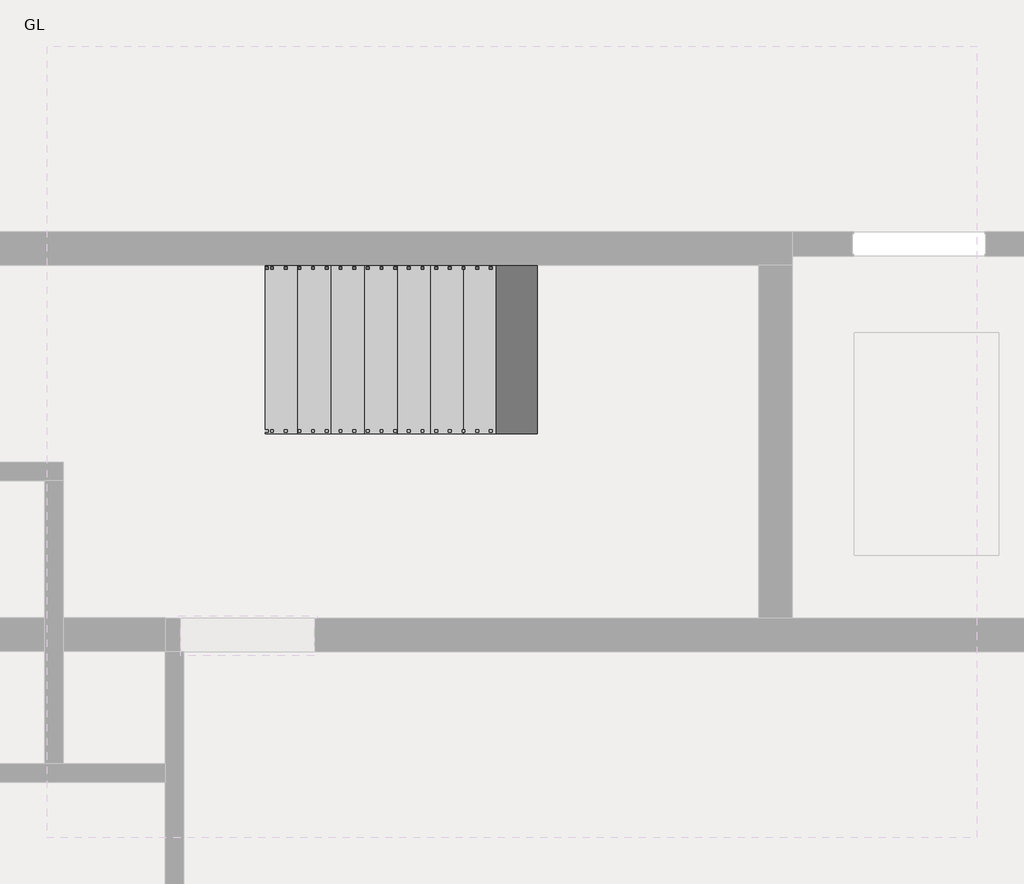
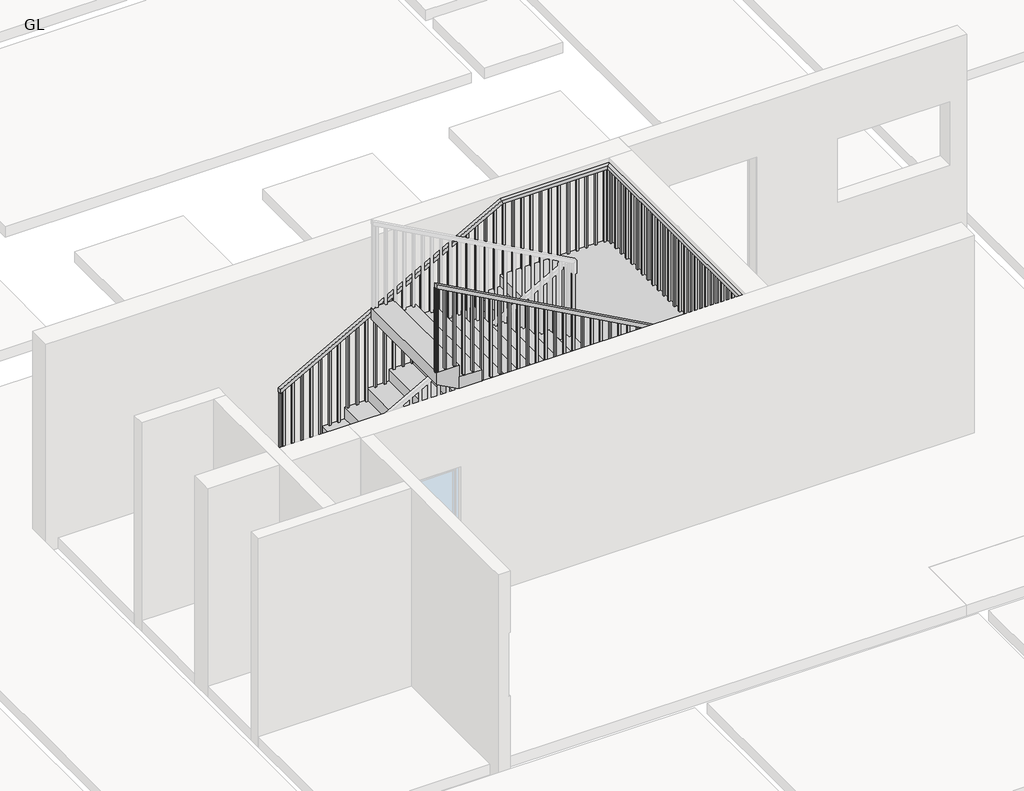
# One storey, part 10 of 14: 1 railing, 1 stair flight.
"""IFC4 building model written with IfcOpenShell, lengths in millimetres."""

from ifc_helpers import new_model, si_unit, frame, origin, place, context, project, spatial, polyline, outline, extrude, faceted_brep, element, save

model = new_model("IFC4")

# Units and contexts
model_context = context("Model", 3, world=origin())
ifc_project = project(units=[si_unit("LENGTHUNIT", "METRE", prefix="MILLI")], contexts=[model_context])

# Site, building, storey
site = spatial("IfcSite", under=ifc_project)
building = spatial("IfcBuilding", under=site)
storey = spatial("IfcBuildingStorey", under=building, Name="GL", Elevation=0.0)

# Railing
placement = place(None, origin())
element("IfcRailing", 1, ObjectType="1100mm", at=placement, inside=storey, context=model_context, shape_type="SolidModel", body=[
    faceted_brep([(-139.7980544, 73095.2178911, 1266.6666667), (-139.7980544, 73095.2178911, 1209.5692982), (-139.7980544, 73045.2178911, 1209.5692982), (-139.7980544, 73045.2178911, 1266.6666667), (2882.8019456, 73095.2178911, 2933.3333333), (2895.6734492, 73095.2178911, 2883.3333333), (2895.6734492, 73045.2178911, 2883.3333333), (2882.8019456, 73045.2178911, 2933.3333333), (4371.714024, 73095.2178911, 2933.3333333), (4371.714024, 73095.2178911, 2883.3333333), (4321.714024, 73045.2178911, 2883.3333333), (4321.714024, 73045.2178911, 2933.3333333), (4371.714024, 69866.5033979, 2933.3333333), (4371.714024, 69866.5033979, 2883.3333333), (4321.714024, 69916.5033979, 2883.3333333), (4321.714024, 69916.5033979, 2933.3333333), (3185.485279, 69866.5033979, 2933.3333333), (3172.6295437, 69866.5033979, 2883.3333333), (3172.6295437, 69916.5033979, 2883.3333333), (3185.485279, 69916.5033979, 2933.3333333), (158.6519456, 69866.5033979, 4600.0), (158.6519456, 69916.5033979, 4600.0), (158.6519456, 69916.5033979, 4542.9212405), (158.6519456, 69866.5033979, 4542.9212405)], [[[0, 1, 2, 3]], [[1, 0, 4, 5]], [[2, 1, 5, 6]], [[3, 2, 6, 7]], [[0, 3, 7, 4]], [[5, 4, 8, 9]], [[6, 5, 9, 10]], [[7, 6, 10, 11]], [[4, 7, 11, 8]], [[9, 8, 12, 13]], [[10, 9, 13, 14]], [[11, 10, 14, 15]], [[8, 11, 15, 12]], [[13, 12, 16, 17]], [[14, 13, 17, 18]], [[15, 14, 18, 19]], [[12, 15, 19, 16]], [[20, 21, 22, 23]], [[17, 16, 20, 23]], [[18, 17, 23, 22]], [[19, 18, 22, 21]], [[16, 19, 21, 20]]]),
    extrude(outline(polyline([(4535.7288621, 171.714024), (4549.4946239, 146.714024), (3333.3333333, 146.714024), (3333.3333333, 171.714024), (4535.7288621, 171.714024)])), frame((0.0, 69879.0033979, 0.0), z_axis=(0.0, 1.0, 0.0), x_axis=(0.0, 0.0, 1.0)), (0.0, 0.0, 1.0), 25.0),
    extrude(outline(polyline([(4466.9000531, 296.714024), (4480.6658149, 271.714024), (3333.3333333, 271.714024), (3333.3333333, 296.714024), (4466.9000531, 296.714024)])), frame((0.0, 69879.0033979, 0.0), z_axis=(0.0, 1.0, 0.0), x_axis=(0.0, 0.0, 1.0)), (0.0, 0.0, 1.0), 25.0),
    extrude(outline(polyline([(4398.0712441, 421.714024), (4411.8370059, 396.714024), (3333.3333333, 396.714024), (3333.3333333, 421.714024), (4398.0712441, 421.714024)])), frame((0.0, 69879.0033979, 0.0), z_axis=(0.0, 1.0, 0.0), x_axis=(0.0, 0.0, 1.0)), (0.0, 0.0, 1.0), 25.0),
    extrude(outline(polyline([(4329.2424351, 546.714024), (4343.0081969, 521.714024), (3166.6666667, 521.714024), (3166.6666667, 546.714024), (4329.2424351, 546.714024)])), frame((0.0, 69879.0033979, 0.0), z_axis=(0.0, 1.0, 0.0), x_axis=(0.0, 0.0, 1.0)), (0.0, 0.0, 1.0), 25.0),
    extrude(outline(polyline([(4260.4136261, 671.714024), (4274.1793879, 646.714024), (3166.6666667, 646.714024), (3166.6666667, 671.714024), (4260.4136261, 671.714024)])), frame((0.0, 69879.0033979, 0.0), z_axis=(0.0, 1.0, 0.0), x_axis=(0.0, 0.0, 1.0)), (0.0, 0.0, 1.0), 25.0),
    extrude(outline(polyline([(4191.5848171, 796.714024), (4205.3505789, 771.714024), (3000.0, 771.714024), (3000.0, 796.714024), (4191.5848171, 796.714024)])), frame((0.0, 69879.0033979, 0.0), z_axis=(0.0, 1.0, 0.0), x_axis=(0.0, 0.0, 1.0)), (0.0, 0.0, 1.0), 25.0),
    extrude(outline(polyline([(4122.7560081, 921.714024), (4136.5217699, 896.714024), (3000.0, 896.714024), (3000.0, 921.714024), (4122.7560081, 921.714024)])), frame((0.0, 69879.0033979, 0.0), z_axis=(0.0, 1.0, 0.0), x_axis=(0.0, 0.0, 1.0)), (0.0, 0.0, 1.0), 25.0),
    extrude(outline(polyline([(4053.9271992, 1046.714024), (4067.6929609, 1021.714024), (3000.0, 1021.714024), (3000.0, 1046.714024), (4053.9271992, 1046.714024)])), frame((0.0, 69879.0033979, 0.0), z_axis=(0.0, 1.0, 0.0), x_axis=(0.0, 0.0, 1.0)), (0.0, 0.0, 1.0), 25.0),
    extrude(outline(polyline([(3985.0983902, 1171.714024), (3998.864152, 1146.714024), (2833.3333333, 1146.714024), (2833.3333333, 1171.714024), (3985.0983902, 1171.714024)])), frame((0.0, 69879.0033979, 0.0), z_axis=(0.0, 1.0, 0.0), x_axis=(0.0, 0.0, 1.0)), (0.0, 0.0, 1.0), 25.0),
    extrude(outline(polyline([(3916.2695812, 1296.714024), (3930.035343, 1271.714024), (2833.3333333, 1271.714024), (2833.3333333, 1296.714024), (3916.2695812, 1296.714024)])), frame((0.0, 69879.0033979, 0.0), z_axis=(0.0, 1.0, 0.0), x_axis=(0.0, 0.0, 1.0)), (0.0, 0.0, 1.0), 25.0),
    extrude(outline(polyline([(3847.4407722, 1421.714024), (3861.206534, 1396.714024), (2666.6666667, 1396.714024), (2666.6666667, 1421.714024), (3847.4407722, 1421.714024)])), frame((0.0, 69879.0033979, 0.0), z_axis=(0.0, 1.0, 0.0), x_axis=(0.0, 0.0, 1.0)), (0.0, 0.0, 1.0), 25.0),
    extrude(outline(polyline([(3778.6119632, 1546.714024), (3792.377725, 1521.714024), (2666.6666667, 1521.714024), (2666.6666667, 1546.714024), (3778.6119632, 1546.714024)])), frame((0.0, 69879.0033979, 0.0), z_axis=(0.0, 1.0, 0.0), x_axis=(0.0, 0.0, 1.0)), (0.0, 0.0, 1.0), 25.0),
    extrude(outline(polyline([(3709.7831542, 1671.714024), (3723.548916, 1646.714024), (2666.6666667, 1646.714024), (2666.6666667, 1671.714024), (3709.7831542, 1671.714024)])), frame((0.0, 69879.0033979, 0.0), z_axis=(0.0, 1.0, 0.0), x_axis=(0.0, 0.0, 1.0)), (0.0, 0.0, 1.0), 25.0),
    extrude(outline(polyline([(3640.9543452, 1796.714024), (3654.720107, 1771.714024), (2500.0, 1771.714024), (2500.0, 1796.714024), (3640.9543452, 1796.714024)])), frame((0.0, 69879.0033979, 0.0), z_axis=(0.0, 1.0, 0.0), x_axis=(0.0, 0.0, 1.0)), (0.0, 0.0, 1.0), 25.0),
    extrude(outline(polyline([(3572.1255362, 1921.714024), (3585.891298, 1896.714024), (2500.0, 1896.714024), (2500.0, 1921.714024), (3572.1255362, 1921.714024)])), frame((0.0, 69879.0033979, 0.0), z_axis=(0.0, 1.0, 0.0), x_axis=(0.0, 0.0, 1.0)), (0.0, 0.0, 1.0), 25.0),
    extrude(outline(polyline([(3503.2967273, 2046.714024), (3517.0624891, 2021.714024), (2333.3333333, 2021.714024), (2333.3333333, 2046.714024), (3503.2967273, 2046.714024)])), frame((0.0, 69879.0033979, 0.0), z_axis=(0.0, 1.0, 0.0), x_axis=(0.0, 0.0, 1.0)), (0.0, 0.0, 1.0), 25.0),
    extrude(outline(polyline([(3434.4679183, 2171.714024), (3448.2336801, 2146.714024), (2333.3333333, 2146.714024), (2333.3333333, 2171.714024), (3434.4679183, 2171.714024)])), frame((0.0, 69879.0033979, 0.0), z_axis=(0.0, 1.0, 0.0), x_axis=(0.0, 0.0, 1.0)), (0.0, 0.0, 1.0), 25.0),
    extrude(outline(polyline([(3365.6391093, 2296.714024), (3379.4048711, 2271.714024), (2166.6666667, 2271.714024), (2166.6666667, 2296.714024), (3365.6391093, 2296.714024)])), frame((0.0, 69879.0033979, 0.0), z_axis=(0.0, 1.0, 0.0), x_axis=(0.0, 0.0, 1.0)), (0.0, 0.0, 1.0), 25.0),
    extrude(outline(polyline([(3296.8103003, 2421.714024), (3310.5760621, 2396.714024), (2166.6666667, 2396.714024), (2166.6666667, 2421.714024), (3296.8103003, 2421.714024)])), frame((0.0, 69879.0033979, 0.0), z_axis=(0.0, 1.0, 0.0), x_axis=(0.0, 0.0, 1.0)), (0.0, 0.0, 1.0), 25.0),
    extrude(outline(polyline([(3227.9814913, 2546.714024), (3241.7472531, 2521.714024), (2166.6666667, 2521.714024), (2166.6666667, 2546.714024), (3227.9814913, 2546.714024)])), frame((0.0, 69879.0033979, 0.0), z_axis=(0.0, 1.0, 0.0), x_axis=(0.0, 0.0, 1.0)), (0.0, 0.0, 1.0), 25.0),
    extrude(outline(polyline([(3159.1526823, 2671.714024), (3172.9184441, 2646.714024), (2000.0, 2646.714024), (2000.0, 2671.714024), (3159.1526823, 2671.714024)])), frame((0.0, 69879.0033979, 0.0), z_axis=(0.0, 1.0, 0.0), x_axis=(0.0, 0.0, 1.0)), (0.0, 0.0, 1.0), 25.0),
    extrude(outline(polyline([(3090.3238733, 2796.714024), (3104.0896351, 2771.714024), (2000.0, 2771.714024), (2000.0, 2796.714024), (3090.3238733, 2796.714024)])), frame((0.0, 69879.0033979, 0.0), z_axis=(0.0, 1.0, 0.0), x_axis=(0.0, 0.0, 1.0)), (0.0, 0.0, 1.0), 25.0),
    extrude(outline(polyline([(3021.4950644, 2921.714024), (3035.2608262, 2896.714024), (1833.3333333, 2896.714024), (1833.3333333, 2921.714024), (3021.4950644, 2921.714024)])), frame((0.0, 69879.0033979, 0.0), z_axis=(0.0, 1.0, 0.0), x_axis=(0.0, 0.0, 1.0)), (0.0, 0.0, 1.0), 25.0),
    extrude(outline(polyline([(2952.6662554, 3046.714024), (2966.4320172, 3021.714024), (1833.3333333, 3021.714024), (1833.3333333, 3046.714024), (2952.6662554, 3046.714024)])), frame((0.0, 69879.0033979, 0.0), z_axis=(0.0, 1.0, 0.0), x_axis=(0.0, 0.0, 1.0)), (0.0, 0.0, 1.0), 25.0),
    extrude(outline(polyline([(2883.8374464, 3171.714024), (2897.6032082, 3146.714024), (1833.3333333, 3146.714024), (1833.3333333, 3171.714024), (2883.8374464, 3171.714024)])), frame((0.0, 69879.0033979, 0.0), z_axis=(0.0, 1.0, 0.0), x_axis=(0.0, 0.0, 1.0)), (0.0, 0.0, 1.0), 25.0),
    extrude(outline(polyline([(3296.714024, 69879.0033979), (3271.714024, 69879.0033979), (3271.714024, 69904.0033979), (3296.714024, 69904.0033979), (3296.714024, 69879.0033979)])), frame((0.0, 0.0, 1833.3333333), z_axis=(0.0, 0.0, 1.0), x_axis=(1.0, 0.0, 0.0)), (0.0, 0.0, 1.0), 1050.0),
    extrude(outline(polyline([(3421.714024, 69879.0033979), (3396.714024, 69879.0033979), (3396.714024, 69904.0033979), (3421.714024, 69904.0033979), (3421.714024, 69879.0033979)])), frame((0.0, 0.0, 1833.3333333), z_axis=(0.0, 0.0, 1.0), x_axis=(1.0, 0.0, 0.0)), (0.0, 0.0, 1.0), 1050.0),
    extrude(outline(polyline([(3546.714024, 69879.0033979), (3521.714024, 69879.0033979), (3521.714024, 69904.0033979), (3546.714024, 69904.0033979), (3546.714024, 69879.0033979)])), frame((0.0, 0.0, 1833.3333333), z_axis=(0.0, 0.0, 1.0), x_axis=(1.0, 0.0, 0.0)), (0.0, 0.0, 1.0), 1050.0),
    extrude(outline(polyline([(3671.714024, 69879.0033979), (3646.714024, 69879.0033979), (3646.714024, 69904.0033979), (3671.714024, 69904.0033979), (3671.714024, 69879.0033979)])), frame((0.0, 0.0, 1833.3333333), z_axis=(0.0, 0.0, 1.0), x_axis=(1.0, 0.0, 0.0)), (0.0, 0.0, 1.0), 1050.0),
    extrude(outline(polyline([(3796.714024, 69879.0033979), (3771.714024, 69879.0033979), (3771.714024, 69904.0033979), (3796.714024, 69904.0033979), (3796.714024, 69879.0033979)])), frame((0.0, 0.0, 1833.3333333), z_axis=(0.0, 0.0, 1.0), x_axis=(1.0, 0.0, 0.0)), (0.0, 0.0, 1.0), 1050.0),
    extrude(outline(polyline([(3921.714024, 69879.0033979), (3896.714024, 69879.0033979), (3896.714024, 69904.0033979), (3921.714024, 69904.0033979), (3921.714024, 69879.0033979)])), frame((0.0, 0.0, 1833.3333333), z_axis=(0.0, 0.0, 1.0), x_axis=(1.0, 0.0, 0.0)), (0.0, 0.0, 1.0), 1050.0),
    extrude(outline(polyline([(4046.714024, 69879.0033979), (4021.714024, 69879.0033979), (4021.714024, 69904.0033979), (4046.714024, 69904.0033979), (4046.714024, 69879.0033979)])), frame((0.0, 0.0, 1833.3333333), z_axis=(0.0, 0.0, 1.0), x_axis=(1.0, 0.0, 0.0)), (0.0, 0.0, 1.0), 1050.0),
    extrude(outline(polyline([(4171.714024, 69879.0033979), (4146.714024, 69879.0033979), (4146.714024, 69904.0033979), (4171.714024, 69904.0033979), (4171.714024, 69879.0033979)])), frame((0.0, 0.0, 1833.3333333), z_axis=(0.0, 0.0, 1.0), x_axis=(1.0, 0.0, 0.0)), (0.0, 0.0, 1.0), 1050.0),
    extrude(outline(polyline([(4296.714024, 69879.0033979), (4271.714024, 69879.0033979), (4271.714024, 69904.0033979), (4296.714024, 69904.0033979), (4296.714024, 69879.0033979)])), frame((0.0, 0.0, 1833.3333333), z_axis=(0.0, 0.0, 1.0), x_axis=(1.0, 0.0, 0.0)), (0.0, 0.0, 1.0), 1050.0),
    extrude(outline(polyline([(4359.214024, 70020.2178911), (4359.214024, 69995.2178911), (4334.214024, 69995.2178911), (4334.214024, 70020.2178911), (4359.214024, 70020.2178911)])), frame((0.0, 0.0, 1833.3333333), z_axis=(0.0, 0.0, 1.0), x_axis=(1.0, 0.0, 0.0)), (0.0, 0.0, 1.0), 1050.0),
    extrude(outline(polyline([(4359.214024, 70145.2178911), (4359.214024, 70120.2178911), (4334.214024, 70120.2178911), (4334.214024, 70145.2178911), (4359.214024, 70145.2178911)])), frame((0.0, 0.0, 1833.3333333), z_axis=(0.0, 0.0, 1.0), x_axis=(1.0, 0.0, 0.0)), (0.0, 0.0, 1.0), 1050.0),
    extrude(outline(polyline([(4359.214024, 70270.2178911), (4359.214024, 70245.2178911), (4334.214024, 70245.2178911), (4334.214024, 70270.2178911), (4359.214024, 70270.2178911)])), frame((0.0, 0.0, 1833.3333333), z_axis=(0.0, 0.0, 1.0), x_axis=(1.0, 0.0, 0.0)), (0.0, 0.0, 1.0), 1050.0),
    extrude(outline(polyline([(4359.214024, 70395.2178911), (4359.214024, 70370.2178911), (4334.214024, 70370.2178911), (4334.214024, 70395.2178911), (4359.214024, 70395.2178911)])), frame((0.0, 0.0, 1833.3333333), z_axis=(0.0, 0.0, 1.0), x_axis=(1.0, 0.0, 0.0)), (0.0, 0.0, 1.0), 1050.0),
    extrude(outline(polyline([(4359.214024, 70520.2178911), (4359.214024, 70495.2178911), (4334.214024, 70495.2178911), (4334.214024, 70520.2178911), (4359.214024, 70520.2178911)])), frame((0.0, 0.0, 1833.3333333), z_axis=(0.0, 0.0, 1.0), x_axis=(1.0, 0.0, 0.0)), (0.0, 0.0, 1.0), 1050.0),
    extrude(outline(polyline([(4359.214024, 70645.2178911), (4359.214024, 70620.2178911), (4334.214024, 70620.2178911), (4334.214024, 70645.2178911), (4359.214024, 70645.2178911)])), frame((0.0, 0.0, 1833.3333333), z_axis=(0.0, 0.0, 1.0), x_axis=(1.0, 0.0, 0.0)), (0.0, 0.0, 1.0), 1050.0),
    extrude(outline(polyline([(4359.214024, 70770.2178911), (4359.214024, 70745.2178911), (4334.214024, 70745.2178911), (4334.214024, 70770.2178911), (4359.214024, 70770.2178911)])), frame((0.0, 0.0, 1833.3333333), z_axis=(0.0, 0.0, 1.0), x_axis=(1.0, 0.0, 0.0)), (0.0, 0.0, 1.0), 1050.0),
    extrude(outline(polyline([(4359.214024, 70895.2178911), (4359.214024, 70870.2178911), (4334.214024, 70870.2178911), (4334.214024, 70895.2178911), (4359.214024, 70895.2178911)])), frame((0.0, 0.0, 1833.3333333), z_axis=(0.0, 0.0, 1.0), x_axis=(1.0, 0.0, 0.0)), (0.0, 0.0, 1.0), 1050.0),
    extrude(outline(polyline([(4359.214024, 71020.2178911), (4359.214024, 70995.2178911), (4334.214024, 70995.2178911), (4334.214024, 71020.2178911), (4359.214024, 71020.2178911)])), frame((0.0, 0.0, 1833.3333333), z_axis=(0.0, 0.0, 1.0), x_axis=(1.0, 0.0, 0.0)), (0.0, 0.0, 1.0), 1050.0),
    extrude(outline(polyline([(4359.214024, 71145.2178911), (4359.214024, 71120.2178911), (4334.214024, 71120.2178911), (4334.214024, 71145.2178911), (4359.214024, 71145.2178911)])), frame((0.0, 0.0, 1833.3333333), z_axis=(0.0, 0.0, 1.0), x_axis=(1.0, 0.0, 0.0)), (0.0, 0.0, 1.0), 1050.0),
    extrude(outline(polyline([(4359.214024, 71270.2178911), (4359.214024, 71245.2178911), (4334.214024, 71245.2178911), (4334.214024, 71270.2178911), (4359.214024, 71270.2178911)])), frame((0.0, 0.0, 1833.3333333), z_axis=(0.0, 0.0, 1.0), x_axis=(1.0, 0.0, 0.0)), (0.0, 0.0, 1.0), 1050.0),
    extrude(outline(polyline([(4359.214024, 71395.2178911), (4359.214024, 71370.2178911), (4334.214024, 71370.2178911), (4334.214024, 71395.2178911), (4359.214024, 71395.2178911)])), frame((0.0, 0.0, 1833.3333333), z_axis=(0.0, 0.0, 1.0), x_axis=(1.0, 0.0, 0.0)), (0.0, 0.0, 1.0), 1050.0),
    extrude(outline(polyline([(4359.214024, 71520.2178911), (4359.214024, 71495.2178911), (4334.214024, 71495.2178911), (4334.214024, 71520.2178911), (4359.214024, 71520.2178911)])), frame((0.0, 0.0, 1833.3333333), z_axis=(0.0, 0.0, 1.0), x_axis=(1.0, 0.0, 0.0)), (0.0, 0.0, 1.0), 1050.0),
    extrude(outline(polyline([(4359.214024, 71645.2178911), (4359.214024, 71620.2178911), (4334.214024, 71620.2178911), (4334.214024, 71645.2178911), (4359.214024, 71645.2178911)])), frame((0.0, 0.0, 1833.3333333), z_axis=(0.0, 0.0, 1.0), x_axis=(1.0, 0.0, 0.0)), (0.0, 0.0, 1.0), 1050.0),
    extrude(outline(polyline([(4359.214024, 71770.2178911), (4359.214024, 71745.2178911), (4334.214024, 71745.2178911), (4334.214024, 71770.2178911), (4359.214024, 71770.2178911)])), frame((0.0, 0.0, 1833.3333333), z_axis=(0.0, 0.0, 1.0), x_axis=(1.0, 0.0, 0.0)), (0.0, 0.0, 1.0), 1050.0),
    extrude(outline(polyline([(4359.214024, 71895.2178911), (4359.214024, 71870.2178911), (4334.214024, 71870.2178911), (4334.214024, 71895.2178911), (4359.214024, 71895.2178911)])), frame((0.0, 0.0, 1833.3333333), z_axis=(0.0, 0.0, 1.0), x_axis=(1.0, 0.0, 0.0)), (0.0, 0.0, 1.0), 1050.0),
    extrude(outline(polyline([(4359.214024, 72020.2178911), (4359.214024, 71995.2178911), (4334.214024, 71995.2178911), (4334.214024, 72020.2178911), (4359.214024, 72020.2178911)])), frame((0.0, 0.0, 1833.3333333), z_axis=(0.0, 0.0, 1.0), x_axis=(1.0, 0.0, 0.0)), (0.0, 0.0, 1.0), 1050.0),
    extrude(outline(polyline([(4359.214024, 72145.2178911), (4359.214024, 72120.2178911), (4334.214024, 72120.2178911), (4334.214024, 72145.2178911), (4359.214024, 72145.2178911)])), frame((0.0, 0.0, 1833.3333333), z_axis=(0.0, 0.0, 1.0), x_axis=(1.0, 0.0, 0.0)), (0.0, 0.0, 1.0), 1050.0),
    extrude(outline(polyline([(4359.214024, 72270.2178911), (4359.214024, 72245.2178911), (4334.214024, 72245.2178911), (4334.214024, 72270.2178911), (4359.214024, 72270.2178911)])), frame((0.0, 0.0, 1833.3333333), z_axis=(0.0, 0.0, 1.0), x_axis=(1.0, 0.0, 0.0)), (0.0, 0.0, 1.0), 1050.0),
    extrude(outline(polyline([(4359.214024, 72395.2178911), (4359.214024, 72370.2178911), (4334.214024, 72370.2178911), (4334.214024, 72395.2178911), (4359.214024, 72395.2178911)])), frame((0.0, 0.0, 1833.3333333), z_axis=(0.0, 0.0, 1.0), x_axis=(1.0, 0.0, 0.0)), (0.0, 0.0, 1.0), 1050.0),
    extrude(outline(polyline([(4359.214024, 72520.2178911), (4359.214024, 72495.2178911), (4334.214024, 72495.2178911), (4334.214024, 72520.2178911), (4359.214024, 72520.2178911)])), frame((0.0, 0.0, 1833.3333333), z_axis=(0.0, 0.0, 1.0), x_axis=(1.0, 0.0, 0.0)), (0.0, 0.0, 1.0), 1050.0),
    extrude(outline(polyline([(4359.214024, 72645.2178911), (4359.214024, 72620.2178911), (4334.214024, 72620.2178911), (4334.214024, 72645.2178911), (4359.214024, 72645.2178911)])), frame((0.0, 0.0, 1833.3333333), z_axis=(0.0, 0.0, 1.0), x_axis=(1.0, 0.0, 0.0)), (0.0, 0.0, 1.0), 1050.0),
    extrude(outline(polyline([(4359.214024, 72770.2178911), (4359.214024, 72745.2178911), (4334.214024, 72745.2178911), (4334.214024, 72770.2178911), (4359.214024, 72770.2178911)])), frame((0.0, 0.0, 1833.3333333), z_axis=(0.0, 0.0, 1.0), x_axis=(1.0, 0.0, 0.0)), (0.0, 0.0, 1.0), 1050.0),
    extrude(outline(polyline([(4359.214024, 72895.2178911), (4359.214024, 72870.2178911), (4334.214024, 72870.2178911), (4334.214024, 72895.2178911), (4359.214024, 72895.2178911)])), frame((0.0, 0.0, 1833.3333333), z_axis=(0.0, 0.0, 1.0), x_axis=(1.0, 0.0, 0.0)), (0.0, 0.0, 1.0), 1050.0),
    extrude(outline(polyline([(4359.214024, 73020.2178911), (4359.214024, 72995.2178911), (4334.214024, 72995.2178911), (4334.214024, 73020.2178911), (4359.214024, 73020.2178911)])), frame((0.0, 0.0, 1833.3333333), z_axis=(0.0, 0.0, 1.0), x_axis=(1.0, 0.0, 0.0)), (0.0, 0.0, 1.0), 1050.0),
    extrude(outline(polyline([(4285.2019456, 73082.7178911), (4310.2019456, 73082.7178911), (4310.2019456, 73057.7178911), (4285.2019456, 73057.7178911), (4285.2019456, 73082.7178911)])), frame((0.0, 0.0, 1833.3333333), z_axis=(0.0, 0.0, 1.0), x_axis=(1.0, 0.0, 0.0)), (0.0, 0.0, 1.0), 1050.0),
    extrude(outline(polyline([(4160.2019456, 73082.7178911), (4185.2019456, 73082.7178911), (4185.2019456, 73057.7178911), (4160.2019456, 73057.7178911), (4160.2019456, 73082.7178911)])), frame((0.0, 0.0, 1833.3333333), z_axis=(0.0, 0.0, 1.0), x_axis=(1.0, 0.0, 0.0)), (0.0, 0.0, 1.0), 1050.0),
    extrude(outline(polyline([(4035.2019456, 73082.7178911), (4060.2019456, 73082.7178911), (4060.2019456, 73057.7178911), (4035.2019456, 73057.7178911), (4035.2019456, 73082.7178911)])), frame((0.0, 0.0, 1833.3333333), z_axis=(0.0, 0.0, 1.0), x_axis=(1.0, 0.0, 0.0)), (0.0, 0.0, 1.0), 1050.0),
    extrude(outline(polyline([(3910.2019456, 73082.7178911), (3935.2019456, 73082.7178911), (3935.2019456, 73057.7178911), (3910.2019456, 73057.7178911), (3910.2019456, 73082.7178911)])), frame((0.0, 0.0, 1833.3333333), z_axis=(0.0, 0.0, 1.0), x_axis=(1.0, 0.0, 0.0)), (0.0, 0.0, 1.0), 1050.0),
    extrude(outline(polyline([(3785.2019456, 73082.7178911), (3810.2019456, 73082.7178911), (3810.2019456, 73057.7178911), (3785.2019456, 73057.7178911), (3785.2019456, 73082.7178911)])), frame((0.0, 0.0, 1833.3333333), z_axis=(0.0, 0.0, 1.0), x_axis=(1.0, 0.0, 0.0)), (0.0, 0.0, 1.0), 1050.0),
    extrude(outline(polyline([(3660.2019456, 73082.7178911), (3685.2019456, 73082.7178911), (3685.2019456, 73057.7178911), (3660.2019456, 73057.7178911), (3660.2019456, 73082.7178911)])), frame((0.0, 0.0, 1833.3333333), z_axis=(0.0, 0.0, 1.0), x_axis=(1.0, 0.0, 0.0)), (0.0, 0.0, 1.0), 1050.0),
    extrude(outline(polyline([(3535.2019456, 73082.7178911), (3560.2019456, 73082.7178911), (3560.2019456, 73057.7178911), (3535.2019456, 73057.7178911), (3535.2019456, 73082.7178911)])), frame((0.0, 0.0, 1833.3333333), z_axis=(0.0, 0.0, 1.0), x_axis=(1.0, 0.0, 0.0)), (0.0, 0.0, 1.0), 1050.0),
    extrude(outline(polyline([(3410.2019456, 73082.7178911), (3435.2019456, 73082.7178911), (3435.2019456, 73057.7178911), (3410.2019456, 73057.7178911), (3410.2019456, 73082.7178911)])), frame((0.0, 0.0, 1833.3333333), z_axis=(0.0, 0.0, 1.0), x_axis=(1.0, 0.0, 0.0)), (0.0, 0.0, 1.0), 1050.0),
    extrude(outline(polyline([(3285.2019456, 73082.7178911), (3310.2019456, 73082.7178911), (3310.2019456, 73057.7178911), (3285.2019456, 73057.7178911), (3285.2019456, 73082.7178911)])), frame((0.0, 0.0, 1833.3333333), z_axis=(0.0, 0.0, 1.0), x_axis=(1.0, 0.0, 0.0)), (0.0, 0.0, 1.0), 1050.0),
    extrude(outline(polyline([(3160.2019456, 73082.7178911), (3185.2019456, 73082.7178911), (3185.2019456, 73057.7178911), (3160.2019456, 73057.7178911), (3160.2019456, 73082.7178911)])), frame((0.0, 0.0, 1833.3333333), z_axis=(0.0, 0.0, 1.0), x_axis=(1.0, 0.0, 0.0)), (0.0, 0.0, 1.0), 1050.0),
    extrude(outline(polyline([(3035.2019456, 73082.7178911), (3060.2019456, 73082.7178911), (3060.2019456, 73057.7178911), (3035.2019456, 73057.7178911), (3035.2019456, 73082.7178911)])), frame((0.0, 0.0, 1833.3333333), z_axis=(0.0, 0.0, 1.0), x_axis=(1.0, 0.0, 0.0)), (0.0, 0.0, 1.0), 1050.0),
    extrude(outline(polyline([(2910.2019456, 73082.7178911), (2935.2019456, 73082.7178911), (2935.2019456, 73057.7178911), (2910.2019456, 73057.7178911), (2910.2019456, 73082.7178911)])), frame((0.0, 0.0, 1833.3333333), z_axis=(0.0, 0.0, 1.0), x_axis=(1.0, 0.0, 0.0)), (0.0, 0.0, 1.0), 1050.0),
    extrude(outline(polyline([(1666.6666667, 2785.2019456), (1666.6666667, 2810.2019456), (2836.2042041, 2810.2019456), (2822.4191626, 2785.2019456), (1666.6666667, 2785.2019456)])), frame((0.0, 73057.7178911, 0.0), z_axis=(0.0, 1.0, 0.0), x_axis=(0.0, 0.0, 1.0)), (0.0, 0.0, 1.0), 25.0),
    extrude(outline(polyline([(1666.6666667, 2660.2019456), (1666.6666667, 2685.2019456), (2767.2789963, 2685.2019456), (2753.4939547, 2660.2019456), (1666.6666667, 2660.2019456)])), frame((0.0, 73057.7178911, 0.0), z_axis=(0.0, 1.0, 0.0), x_axis=(0.0, 0.0, 1.0)), (0.0, 0.0, 1.0), 25.0),
    extrude(outline(polyline([(1500.0, 2535.2019456), (1500.0, 2560.2019456), (2698.3537884, 2560.2019456), (2684.5687468, 2535.2019456), (1500.0, 2535.2019456)])), frame((0.0, 73057.7178911, 0.0), z_axis=(0.0, 1.0, 0.0), x_axis=(0.0, 0.0, 1.0)), (0.0, 0.0, 1.0), 25.0),
    extrude(outline(polyline([(1500.0, 2410.2019456), (1500.0, 2435.2019456), (2629.4285805, 2435.2019456), (2615.6435389, 2410.2019456), (1500.0, 2410.2019456)])), frame((0.0, 73057.7178911, 0.0), z_axis=(0.0, 1.0, 0.0), x_axis=(0.0, 0.0, 1.0)), (0.0, 0.0, 1.0), 25.0),
    extrude(outline(polyline([(1500.0, 2285.2019456), (1500.0, 2310.2019456), (2560.5033726, 2310.2019456), (2546.718331, 2285.2019456), (1500.0, 2285.2019456)])), frame((0.0, 73057.7178911, 0.0), z_axis=(0.0, 1.0, 0.0), x_axis=(0.0, 0.0, 1.0)), (0.0, 0.0, 1.0), 25.0),
    extrude(outline(polyline([(1333.3333333, 2160.2019456), (1333.3333333, 2185.2019456), (2491.5781647, 2185.2019456), (2477.7931232, 2160.2019456), (1333.3333333, 2160.2019456)])), frame((0.0, 73057.7178911, 0.0), z_axis=(0.0, 1.0, 0.0), x_axis=(0.0, 0.0, 1.0)), (0.0, 0.0, 1.0), 25.0),
    extrude(outline(polyline([(1333.3333333, 2035.2019456), (1333.3333333, 2060.2019456), (2422.6529569, 2060.2019456), (2408.8679153, 2035.2019456), (1333.3333333, 2035.2019456)])), frame((0.0, 73057.7178911, 0.0), z_axis=(0.0, 1.0, 0.0), x_axis=(0.0, 0.0, 1.0)), (0.0, 0.0, 1.0), 25.0),
    extrude(outline(polyline([(1166.6666667, 1910.2019456), (1166.6666667, 1935.2019456), (2353.727749, 1935.2019456), (2339.9427074, 1910.2019456), (1166.6666667, 1910.2019456)])), frame((0.0, 73057.7178911, 0.0), z_axis=(0.0, 1.0, 0.0), x_axis=(0.0, 0.0, 1.0)), (0.0, 0.0, 1.0), 25.0),
    extrude(outline(polyline([(1166.6666667, 1785.2019456), (1166.6666667, 1810.2019456), (2284.8025411, 1810.2019456), (2271.0174995, 1785.2019456), (1166.6666667, 1785.2019456)])), frame((0.0, 73057.7178911, 0.0), z_axis=(0.0, 1.0, 0.0), x_axis=(0.0, 0.0, 1.0)), (0.0, 0.0, 1.0), 25.0),
    extrude(outline(polyline([(1000.0, 1660.2019456), (1000.0, 1685.2019456), (2215.8773332, 1685.2019456), (2202.0922917, 1660.2019456), (1000.0, 1660.2019456)])), frame((0.0, 73057.7178911, 0.0), z_axis=(0.0, 1.0, 0.0), x_axis=(0.0, 0.0, 1.0)), (0.0, 0.0, 1.0), 25.0),
    extrude(outline(polyline([(1000.0, 1535.2019456), (1000.0, 1560.2019456), (2146.9521254, 1560.2019456), (2133.1670838, 1535.2019456), (1000.0, 1535.2019456)])), frame((0.0, 73057.7178911, 0.0), z_axis=(0.0, 1.0, 0.0), x_axis=(0.0, 0.0, 1.0)), (0.0, 0.0, 1.0), 25.0),
    extrude(outline(polyline([(1000.0, 1410.2019456), (1000.0, 1435.2019456), (2078.0269175, 1435.2019456), (2064.2418759, 1410.2019456), (1000.0, 1410.2019456)])), frame((0.0, 73057.7178911, 0.0), z_axis=(0.0, 1.0, 0.0), x_axis=(0.0, 0.0, 1.0)), (0.0, 0.0, 1.0), 25.0),
    extrude(outline(polyline([(833.3333333, 1285.2019456), (833.3333333, 1310.2019456), (2009.1017096, 1310.2019456), (1995.316668, 1285.2019456), (833.3333333, 1285.2019456)])), frame((0.0, 73057.7178911, 0.0), z_axis=(0.0, 1.0, 0.0), x_axis=(0.0, 0.0, 1.0)), (0.0, 0.0, 1.0), 25.0),
    extrude(outline(polyline([(833.3333333, 1160.2019456), (833.3333333, 1185.2019456), (1940.1765017, 1185.2019456), (1926.3914601, 1160.2019456), (833.3333333, 1160.2019456)])), frame((0.0, 73057.7178911, 0.0), z_axis=(0.0, 1.0, 0.0), x_axis=(0.0, 0.0, 1.0)), (0.0, 0.0, 1.0), 25.0),
    extrude(outline(polyline([(666.6666667, 1035.2019456), (666.6666667, 1060.2019456), (1871.2512938, 1060.2019456), (1857.4662523, 1035.2019456), (666.6666667, 1035.2019456)])), frame((0.0, 73057.7178911, 0.0), z_axis=(0.0, 1.0, 0.0), x_axis=(0.0, 0.0, 1.0)), (0.0, 0.0, 1.0), 25.0),
    extrude(outline(polyline([(666.6666667, 910.2019456), (666.6666667, 935.2019456), (1802.326086, 935.2019456), (1788.5410444, 910.2019456), (666.6666667, 910.2019456)])), frame((0.0, 73057.7178911, 0.0), z_axis=(0.0, 1.0, 0.0), x_axis=(0.0, 0.0, 1.0)), (0.0, 0.0, 1.0), 25.0),
    extrude(outline(polyline([(666.6666667, 785.2019456), (666.6666667, 810.2019456), (1733.4008781, 810.2019456), (1719.6158365, 785.2019456), (666.6666667, 785.2019456)])), frame((0.0, 73057.7178911, 0.0), z_axis=(0.0, 1.0, 0.0), x_axis=(0.0, 0.0, 1.0)), (0.0, 0.0, 1.0), 25.0),
    extrude(outline(polyline([(500.0, 660.2019456), (500.0, 685.2019456), (1664.4756702, 685.2019456), (1650.6906286, 660.2019456), (500.0, 660.2019456)])), frame((0.0, 73057.7178911, 0.0), z_axis=(0.0, 1.0, 0.0), x_axis=(0.0, 0.0, 1.0)), (0.0, 0.0, 1.0), 25.0),
    extrude(outline(polyline([(500.0, 535.2019456), (500.0, 560.2019456), (1595.5504623, 560.2019456), (1581.7654208, 535.2019456), (500.0, 535.2019456)])), frame((0.0, 73057.7178911, 0.0), z_axis=(0.0, 1.0, 0.0), x_axis=(0.0, 0.0, 1.0)), (0.0, 0.0, 1.0), 25.0),
    extrude(outline(polyline([(333.3333333, 410.2019456), (333.3333333, 435.2019456), (1526.6252544, 435.2019456), (1512.8402129, 410.2019456), (333.3333333, 410.2019456)])), frame((0.0, 73057.7178911, 0.0), z_axis=(0.0, 1.0, 0.0), x_axis=(0.0, 0.0, 1.0)), (0.0, 0.0, 1.0), 25.0),
    extrude(outline(polyline([(333.3333333, 285.2019456), (333.3333333, 310.2019456), (1457.7000466, 310.2019456), (1443.915005, 285.2019456), (333.3333333, 285.2019456)])), frame((0.0, 73057.7178911, 0.0), z_axis=(0.0, 1.0, 0.0), x_axis=(0.0, 0.0, 1.0)), (0.0, 0.0, 1.0), 25.0),
    extrude(outline(polyline([(333.3333333, 160.2019456), (333.3333333, 185.2019456), (1388.7748387, 185.2019456), (1374.9897971, 160.2019456), (333.3333333, 160.2019456)])), frame((0.0, 73057.7178911, 0.0), z_axis=(0.0, 1.0, 0.0), x_axis=(0.0, 0.0, 1.0)), (0.0, 0.0, 1.0), 25.0),
    extrude(outline(polyline([(166.6666667, 35.2019456), (166.6666667, 60.2019456), (1319.8496308, 60.2019456), (1306.0645892, 35.2019456), (166.6666667, 35.2019456)])), frame((0.0, 73057.7178911, 0.0), z_axis=(0.0, 1.0, 0.0), x_axis=(0.0, 0.0, 1.0)), (0.0, 0.0, 1.0), 25.0),
    extrude(outline(polyline([(166.6666667, -89.7980544), (166.6666667, -64.7980544), (1250.9244229, -64.7980544), (1237.1393814, -89.7980544), (166.6666667, -89.7980544)])), frame((0.0, 73057.7178911, 0.0), z_axis=(0.0, 1.0, 0.0), x_axis=(0.0, 0.0, 1.0)), (0.0, 0.0, 1.0), 25.0),
    extrude(outline(polyline([(4359.214024, 69904.0033979), (4359.214024, 69879.0033979), (4334.214024, 69879.0033979), (4334.214024, 69904.0033979), (4359.214024, 69904.0033979)])), frame((0.0, 0.0, 1833.3333333), z_axis=(0.0, 0.0, 1.0), x_axis=(1.0, 0.0, 0.0)), (0.0, 0.0, 1.0), 1050.0),
    extrude(outline(polyline([(4334.214024, 73082.7178911), (4359.214024, 73082.7178911), (4359.214024, 73057.7178911), (4334.214024, 73057.7178911), (4334.214024, 73082.7178911)])), frame((0.0, 0.0, 1833.3333333), z_axis=(0.0, 0.0, 1.0), x_axis=(1.0, 0.0, 0.0)), (0.0, 0.0, 1.0), 1050.0),
    extrude(outline(polyline([(4529.1554787, 183.6519456), (4542.9212405, 158.6519456), (3333.3333333, 158.6519456), (3333.3333333, 183.6519456), (4529.1554787, 183.6519456)])), frame((0.0, 69879.0033979, 0.0), z_axis=(0.0, 1.0, 0.0), x_axis=(0.0, 0.0, 1.0)), (0.0, 0.0, 1.0), 25.0),
    extrude(outline(polyline([(166.6666667, -139.7980544), (166.6666667, -114.7980544), (1223.3543398, -114.7980544), (1209.5692982, -139.7980544), (166.6666667, -139.7980544)])), frame((0.0, 73057.7178911, 0.0), z_axis=(0.0, 1.0, 0.0), x_axis=(0.0, 0.0, 1.0)), (0.0, 0.0, 1.0), 25.0),
])

# Stair flight
element("IfcStairFlight", 2, ObjectType="1mm_Tread-150mm_Depth", at=placement, inside=storey, context=model_context, shape_type="SolidModel", body=[
    faceted_brep([(158.6519456, 73095.6178911, 165.6666667), (-139.7980544, 73095.6178911, 165.6666667), (-139.7980544, 71554.9236123, 165.6666667), (158.6519456, 71554.9236123, 165.6666667), (158.6519456, 73095.6178911, 15.6666667), (-139.7980544, 73095.6178911, 15.6666667), (-139.7980544, 71554.9236123, 15.6666667), (158.6519456, 71554.9236123, 15.6666667), (158.6519456, 73095.6178911, 332.3333333), (158.6519456, 71554.9236123, 332.3333333), (197.2191513, 71554.9236123, 332.3333333), (463.4519456, 71554.9236123, 332.3333333), (463.4519456, 73095.6178911, 332.3333333), (197.2191513, 73095.6178911, 332.3333333), (463.4519456, 73095.6178911, 162.2625559), (197.2191513, 73095.6178911, 15.6666667), (197.2191513, 71554.9236123, 15.6666667), (463.4519456, 71554.9236123, 162.2625559), (768.2519456, 73095.6178911, 499.0), (463.4519456, 73095.6178911, 499.0), (463.4519456, 71554.9236123, 499.0), (768.2519456, 71554.9236123, 499.0), (768.2519456, 73095.6178911, 330.0947237), (768.2519456, 71554.9236123, 330.0947237), (1073.0519456, 73095.6178911, 665.6666667), (768.2519456, 73095.6178911, 665.6666667), (768.2519456, 71554.9236123, 665.6666667), (1073.0519456, 71554.9236123, 665.6666667), (1073.0519456, 73095.6178911, 497.9268915), (1073.0519456, 71554.9236123, 497.9268915), (1371.5019456, 73095.6178911, 832.3333333), (1073.0519456, 73095.6178911, 832.3333333), (1073.0519456, 71554.9236123, 832.3333333), (1371.5019456, 71554.9236123, 832.3333333), (1371.5019456, 73095.6178911, 662.2625559), (1371.5019456, 71554.9236123, 662.2625559), (1676.3019456, 73095.6178911, 999.0), (1371.5019456, 73095.6178911, 999.0), (1371.5019456, 71554.9236123, 999.0), (1676.3019456, 71554.9236123, 999.0), (1676.3019456, 73095.6178911, 830.0947237), (1676.3019456, 71554.9236123, 830.0947237), (1973.4665328, 73095.6178911, 1165.6666667), (1676.3019456, 73095.6178911, 1165.6666667), (1676.3019456, 71554.9236123, 1165.6666667), (1973.4665328, 71554.9236123, 1165.6666667), (1973.4665328, 73095.6178911, 993.7226006), (1973.4665328, 71554.9236123, 993.7226006), (2266.8519456, 73095.6178911, 1332.3333333), (1973.4665328, 73095.6178911, 1332.3333333), (1973.4665328, 71554.9236123, 1332.3333333), (2266.8519456, 71554.9236123, 1332.3333333), (2266.8519456, 73095.6178911, 1155.2695489), (2266.8519456, 71554.9236123, 1155.2695489), (2584.3519456, 73095.6178911, 1499.0), (2266.8519456, 73095.6178911, 1499.0), (2266.8519456, 71554.9236123, 1499.0), (2584.3519456, 71554.9236123, 1499.0), (2584.3519456, 73095.6178911, 1330.0947237), (2584.3519456, 71554.9236123, 1330.0947237), (2882.8019456, 73095.6178911, 1665.6666667), (2584.3519456, 73095.6178911, 1665.6666667), (2584.3519456, 71554.9236123, 1665.6666667), (2882.8019456, 71554.9236123, 1665.6666667), (2882.8019456, 73095.6178911, 1494.430388), (3224.0524846, 71554.9236123, 1682.3333333), (2882.8019456, 71554.9236123, 1682.3333333), (2882.8019456, 69866.1033979, 1832.3333333), (4372.114024, 69866.1033979, 1832.3333333), (4372.114024, 73095.6178911, 1832.3333333), (3224.0524846, 73095.6178911, 1832.3333333), (2882.8019456, 73095.6178911, 1832.3333333), (2882.8019456, 71554.9236123, 1832.3333333), (2882.8019456, 71415.2236123, 1832.3333333), (2882.8019456, 69866.1033979, 1682.3333333), (4372.114024, 69866.1033979, 1682.3333333), (4372.114024, 73095.6178911, 1682.3333333), (3224.0524846, 73095.6178911, 1682.3333333), (2882.8019456, 71415.2236123, 1682.3333333), (2882.8019456, 69866.1033979, 1999.0), (2882.8019456, 71415.2236123, 1999.0), (2844.2051871, 71415.2236123, 1999.0), (2584.3519456, 71415.2236123, 1999.0), (2584.3519456, 69866.1033979, 1999.0), (2844.2051871, 69866.1033979, 1999.0), (2584.3519456, 69866.1033979, 1825.5416284), (2844.2051871, 69866.1033979, 1682.3333333), (2844.2051871, 71415.2236123, 1682.3333333), (2584.3519456, 71415.2236123, 1825.5416284), (2266.8519456, 69866.1033979, 2165.6666667), (2584.3519456, 69866.1033979, 2165.6666667), (2584.3519456, 71415.2236123, 2165.6666667), (2266.8519456, 71415.2236123, 2165.6666667), (2266.8519456, 69866.1033979, 2000.5197561), (2266.8519456, 71415.2236123, 2000.5197561), (1973.4665328, 69866.1033979, 2332.3333333), (2266.8519456, 69866.1033979, 2332.3333333), (2266.8519456, 71415.2236123, 2332.3333333), (1973.4665328, 71415.2236123, 2332.3333333), (1973.4665328, 69866.1033979, 2162.2080404), (1973.4665328, 71415.2236123, 2162.2080404), (1676.3019456, 69866.1033979, 2499.0), (1973.4665328, 69866.1033979, 2499.0), (1973.4665328, 71415.2236123, 2499.0), (1676.3019456, 71415.2236123, 2499.0), (1676.3019456, 69866.1033979, 2325.9790737), (1676.3019456, 71415.2236123, 2325.9790737), (1371.5019456, 69866.1033979, 2665.6666667), (1676.3019456, 69866.1033979, 2665.6666667), (1676.3019456, 71415.2236123, 2665.6666667), (1371.5019456, 71415.2236123, 2665.6666667), (1371.5019456, 69866.1033979, 2493.9580763), (1371.5019456, 71415.2236123, 2493.9580763), (1073.0519456, 69866.1033979, 2832.3333333), (1371.5019456, 69866.1033979, 2832.3333333), (1371.5019456, 71415.2236123, 2832.3333333), (1073.0519456, 71415.2236123, 2832.3333333), (1073.0519456, 69866.1033979, 2658.4375164), (1073.0519456, 71415.2236123, 2658.4375164), (768.2519456, 69866.1033979, 2999.0), (1073.0519456, 69866.1033979, 2999.0), (1073.0519456, 71415.2236123, 2999.0), (768.2519456, 71415.2236123, 2999.0), (768.2519456, 69866.1033979, 2826.416519), (768.2519456, 71415.2236123, 2826.416519), (463.4519456, 69866.1033979, 3165.6666667), (768.2519456, 69866.1033979, 3165.6666667), (768.2519456, 71415.2236123, 3165.6666667), (463.4519456, 71415.2236123, 3165.6666667), (463.4519456, 69866.1033979, 2994.3955217), (463.4519456, 71415.2236123, 2994.3955217), (158.6519456, 69866.1033979, 3332.3333333), (463.4519456, 69866.1033979, 3332.3333333), (463.4519456, 71415.2236123, 3332.3333333), (158.6519456, 71415.2236123, 3332.3333333), (158.6519456, 69866.1033979, 3162.3745243), (158.6519456, 71415.2236123, 3162.3745243)], [[[0, 1, 2, 3]], [[1, 0, 4, 5]], [[2, 1, 5, 6]], [[3, 2, 6, 7]], [[8, 9, 10, 11, 12, 13]], [[0, 8, 13, 12, 14, 15, 4]], [[0, 3, 9, 8]], [[9, 3, 7, 16, 17, 11, 10]], [[18, 19, 20, 21]], [[19, 18, 22, 14, 12]], [[12, 11, 20, 19]], [[21, 20, 11, 17, 23]], [[24, 25, 26, 27]], [[25, 24, 28, 22, 18]], [[18, 21, 26, 25]], [[27, 26, 21, 23, 29]], [[30, 31, 32, 33]], [[31, 30, 34, 28, 24]], [[24, 27, 32, 31]], [[33, 32, 27, 29, 35]], [[36, 37, 38, 39]], [[37, 36, 40, 34, 30]], [[30, 33, 38, 37]], [[39, 38, 33, 35, 41]], [[42, 43, 44, 45]], [[43, 42, 46, 40, 36]], [[36, 39, 44, 43]], [[45, 44, 39, 41, 47]], [[48, 49, 50, 51]], [[49, 48, 52, 46, 42]], [[42, 45, 50, 49]], [[51, 50, 45, 47, 53]], [[54, 55, 56, 57]], [[55, 54, 58, 52, 48]], [[48, 51, 56, 55]], [[57, 56, 51, 53, 59]], [[60, 61, 62, 63]], [[61, 60, 64, 58, 54]], [[54, 57, 62, 61]], [[63, 62, 57, 59, 65, 66]], [[67, 68, 69, 70, 71, 72, 73]], [[68, 67, 74, 75]], [[69, 68, 75, 76]], [[60, 71, 70, 69, 76, 77, 64]], [[60, 63, 66, 72, 71]], [[73, 72, 66, 78]], [[79, 80, 81, 82, 83, 84]], [[67, 79, 84, 83, 85, 86, 74]], [[67, 73, 80, 79]], [[80, 73, 78, 87, 88, 82, 81]], [[89, 90, 91, 92]], [[90, 89, 93, 85, 83]], [[83, 82, 91, 90]], [[92, 91, 82, 88, 94]], [[95, 96, 97, 98]], [[96, 95, 99, 93, 89]], [[89, 92, 97, 96]], [[98, 97, 92, 94, 100]], [[101, 102, 103, 104]], [[102, 101, 105, 99, 95]], [[95, 98, 103, 102]], [[104, 103, 98, 100, 106]], [[107, 108, 109, 110]], [[108, 107, 111, 105, 101]], [[101, 104, 109, 108]], [[110, 109, 104, 106, 112]], [[113, 114, 115, 116]], [[114, 113, 117, 111, 107]], [[107, 110, 115, 114]], [[116, 115, 110, 112, 118]], [[119, 120, 121, 122]], [[120, 119, 123, 117, 113]], [[113, 116, 121, 120]], [[122, 121, 116, 118, 124]], [[125, 126, 127, 128]], [[126, 125, 129, 123, 119]], [[119, 122, 127, 126]], [[128, 127, 122, 124, 130]], [[131, 132, 133, 134]], [[132, 131, 135, 129, 125]], [[125, 128, 133, 132]], [[134, 133, 128, 130, 136]], [[131, 134, 136, 135]], [[15, 16, 7, 6, 5, 4]], [[16, 15, 14, 22, 28, 34, 40, 46, 52, 58, 64, 77, 65, 59, 53, 47, 41, 35, 29, 23, 17]], [[65, 77, 76, 75, 74, 86, 87, 78, 66]], [[87, 86, 85, 93, 99, 105, 111, 117, 123, 129, 135, 136, 130, 124, 118, 112, 106, 100, 94, 88]]]),
    extrude(outline(polyline([(158.6519456, 73095.6178911), (158.6519456, 71554.9236123), (-139.7980544, 71554.9236123), (-139.7980544, 73095.6178911), (158.6519456, 73095.6178911)])), frame((0.0, 0.0, 165.6666667), z_axis=(0.0, 0.0, 1.0), x_axis=(1.0, 0.0, 0.0)), (0.0, 0.0, 1.0), 1.0),
    extrude(outline(polyline([(463.4519456, 73095.6178911), (463.4519456, 71554.9236123), (158.6519456, 71554.9236123), (158.6519456, 73095.6178911), (463.4519456, 73095.6178911)])), frame((0.0, 0.0, 332.3333333), z_axis=(0.0, 0.0, 1.0), x_axis=(1.0, 0.0, 0.0)), (0.0, 0.0, 1.0), 1.0),
    extrude(outline(polyline([(768.2519456, 73095.6178911), (768.2519456, 71554.9236123), (463.4519456, 71554.9236123), (463.4519456, 73095.6178911), (768.2519456, 73095.6178911)])), frame((0.0, 0.0, 499.0), z_axis=(0.0, 0.0, 1.0), x_axis=(1.0, 0.0, 0.0)), (0.0, 0.0, 1.0), 1.0),
    extrude(outline(polyline([(1073.0519456, 73095.6178911), (1073.0519456, 71554.9236123), (768.2519456, 71554.9236123), (768.2519456, 73095.6178911), (1073.0519456, 73095.6178911)])), frame((0.0, 0.0, 665.6666667), z_axis=(0.0, 0.0, 1.0), x_axis=(1.0, 0.0, 0.0)), (0.0, 0.0, 1.0), 1.0),
    extrude(outline(polyline([(1371.5019456, 73095.6178911), (1371.5019456, 71554.9236123), (1073.0519456, 71554.9236123), (1073.0519456, 73095.6178911), (1371.5019456, 73095.6178911)])), frame((0.0, 0.0, 832.3333333), z_axis=(0.0, 0.0, 1.0), x_axis=(1.0, 0.0, 0.0)), (0.0, 0.0, 1.0), 1.0),
    extrude(outline(polyline([(1676.3019456, 73095.6178911), (1676.3019456, 71554.9236123), (1371.5019456, 71554.9236123), (1371.5019456, 73095.6178911), (1676.3019456, 73095.6178911)])), frame((0.0, 0.0, 999.0), z_axis=(0.0, 0.0, 1.0), x_axis=(1.0, 0.0, 0.0)), (0.0, 0.0, 1.0), 1.0),
    extrude(outline(polyline([(1973.4665328, 73095.6178911), (1973.4665328, 71554.9236123), (1676.3019456, 71554.9236123), (1676.3019456, 73095.6178911), (1973.4665328, 73095.6178911)])), frame((0.0, 0.0, 1165.6666667), z_axis=(0.0, 0.0, 1.0), x_axis=(1.0, 0.0, 0.0)), (0.0, 0.0, 1.0), 1.0),
    extrude(outline(polyline([(2266.8519456, 73095.6178911), (2266.8519456, 71554.9236123), (1973.4665328, 71554.9236123), (1973.4665328, 73095.6178911), (2266.8519456, 73095.6178911)])), frame((0.0, 0.0, 1332.3333333), z_axis=(0.0, 0.0, 1.0), x_axis=(1.0, 0.0, 0.0)), (0.0, 0.0, 1.0), 1.0),
    extrude(outline(polyline([(2584.3519456, 73095.6178911), (2584.3519456, 71554.9236123), (2266.8519456, 71554.9236123), (2266.8519456, 73095.6178911), (2584.3519456, 73095.6178911)])), frame((0.0, 0.0, 1499.0), z_axis=(0.0, 0.0, 1.0), x_axis=(1.0, 0.0, 0.0)), (0.0, 0.0, 1.0), 1.0),
    extrude(outline(polyline([(2882.8019456, 73095.6178911), (2882.8019456, 71554.9236123), (2584.3519456, 71554.9236123), (2584.3519456, 73095.6178911), (2882.8019456, 73095.6178911)])), frame((0.0, 0.0, 1665.6666667), z_axis=(0.0, 0.0, 1.0), x_axis=(1.0, 0.0, 0.0)), (0.0, 0.0, 1.0), 1.0),
    extrude(outline(polyline([(2882.8019456, 69866.1033979), (2882.8019456, 71415.2236123), (2882.8019456, 71554.9236123), (2882.8019456, 73095.6178911), (4372.114024, 73095.6178911), (4372.114024, 69866.1033979), (2882.8019456, 69866.1033979)])), frame((0.0, 0.0, 1832.3333333), z_axis=(0.0, 0.0, 1.0), x_axis=(1.0, 0.0, 0.0)), (0.0, 0.0, 1.0), 1.0),
    extrude(outline(polyline([(2584.3519456, 69866.1033979), (2584.3519456, 71415.2236123), (2882.8019456, 71415.2236123), (2882.8019456, 69866.1033979), (2584.3519456, 69866.1033979)])), frame((0.0, 0.0, 1999.0), z_axis=(0.0, 0.0, 1.0), x_axis=(1.0, 0.0, 0.0)), (0.0, 0.0, 1.0), 1.0),
    extrude(outline(polyline([(2266.8519456, 69866.1033979), (2266.8519456, 71415.2236123), (2584.3519456, 71415.2236123), (2584.3519456, 69866.1033979), (2266.8519456, 69866.1033979)])), frame((0.0, 0.0, 2165.6666667), z_axis=(0.0, 0.0, 1.0), x_axis=(1.0, 0.0, 0.0)), (0.0, 0.0, 1.0), 1.0),
    extrude(outline(polyline([(1973.4665328, 69866.1033979), (1973.4665328, 71415.2236123), (2266.8519456, 71415.2236123), (2266.8519456, 69866.1033979), (1973.4665328, 69866.1033979)])), frame((0.0, 0.0, 2332.3333333), z_axis=(0.0, 0.0, 1.0), x_axis=(1.0, 0.0, 0.0)), (0.0, 0.0, 1.0), 1.0),
    extrude(outline(polyline([(1676.3019456, 69866.1033979), (1676.3019456, 71415.2236123), (1973.4665328, 71415.2236123), (1973.4665328, 69866.1033979), (1676.3019456, 69866.1033979)])), frame((0.0, 0.0, 2499.0), z_axis=(0.0, 0.0, 1.0), x_axis=(1.0, 0.0, 0.0)), (0.0, 0.0, 1.0), 1.0),
    extrude(outline(polyline([(1371.5019456, 69866.1033979), (1371.5019456, 71415.2236123), (1676.3019456, 71415.2236123), (1676.3019456, 69866.1033979), (1371.5019456, 69866.1033979)])), frame((0.0, 0.0, 2665.6666667), z_axis=(0.0, 0.0, 1.0), x_axis=(1.0, 0.0, 0.0)), (0.0, 0.0, 1.0), 1.0),
    extrude(outline(polyline([(1073.0519456, 69866.1033979), (1073.0519456, 71415.2236123), (1371.5019456, 71415.2236123), (1371.5019456, 69866.1033979), (1073.0519456, 69866.1033979)])), frame((0.0, 0.0, 2832.3333333), z_axis=(0.0, 0.0, 1.0), x_axis=(1.0, 0.0, 0.0)), (0.0, 0.0, 1.0), 1.0),
    extrude(outline(polyline([(768.2519456, 69866.1033979), (768.2519456, 71415.2236123), (1073.0519456, 71415.2236123), (1073.0519456, 69866.1033979), (768.2519456, 69866.1033979)])), frame((0.0, 0.0, 2999.0), z_axis=(0.0, 0.0, 1.0), x_axis=(1.0, 0.0, 0.0)), (0.0, 0.0, 1.0), 1.0),
    extrude(outline(polyline([(463.4519456, 69866.1033979), (463.4519456, 71415.2236123), (768.2519456, 71415.2236123), (768.2519456, 69866.1033979), (463.4519456, 69866.1033979)])), frame((0.0, 0.0, 3165.6666667), z_axis=(0.0, 0.0, 1.0), x_axis=(1.0, 0.0, 0.0)), (0.0, 0.0, 1.0), 1.0),
    extrude(outline(polyline([(158.6519456, 69866.1033979), (158.6519456, 71415.2236123), (463.4519456, 71415.2236123), (463.4519456, 69866.1033979), (158.6519456, 69866.1033979)])), frame((0.0, 0.0, 3332.3333333), z_axis=(0.0, 0.0, 1.0), x_axis=(1.0, 0.0, 0.0)), (0.0, 0.0, 1.0), 1.0),
])

save(model, "model.ifc")

# Revit data of these elements
# Type "1100mm"
#   built-in parameter 1008612 = 0.019685 (stored number, unit not read)
#   built-in parameter 1008611 = 0.019685 (stored number, unit not read)
#   built-in parameter 1008609 = 0.902231 (stored number, unit not read)
#   built-in parameter 1008604 = 0.19685 (stored number, unit not read)
#   built-in parameter 1008603 = 0.164042 (stored number, unit not read)
#   Railing Height = 3.608924 ft
#   built-in parameter 1008630 = 2
#   built-in parameter 1008610 = 2
#   built-in parameter 1008608 = 1
#   built-in parameter 1008618 = Baluster_Square : 25mm
# Element 1 (IfcRailing, "1100mm")
#   Phase Created = New Construction
# Element 2 (IfcStairFlight, "1mm_Tread-150mm_Depth")
#   Phase Created = New Construction
#   Materials on its faces: "STAIRCASE"
# Materials
#   "STAIRCASE": class "Generic", colour RGB 120 120 120, transparency 0, Cost = 0
